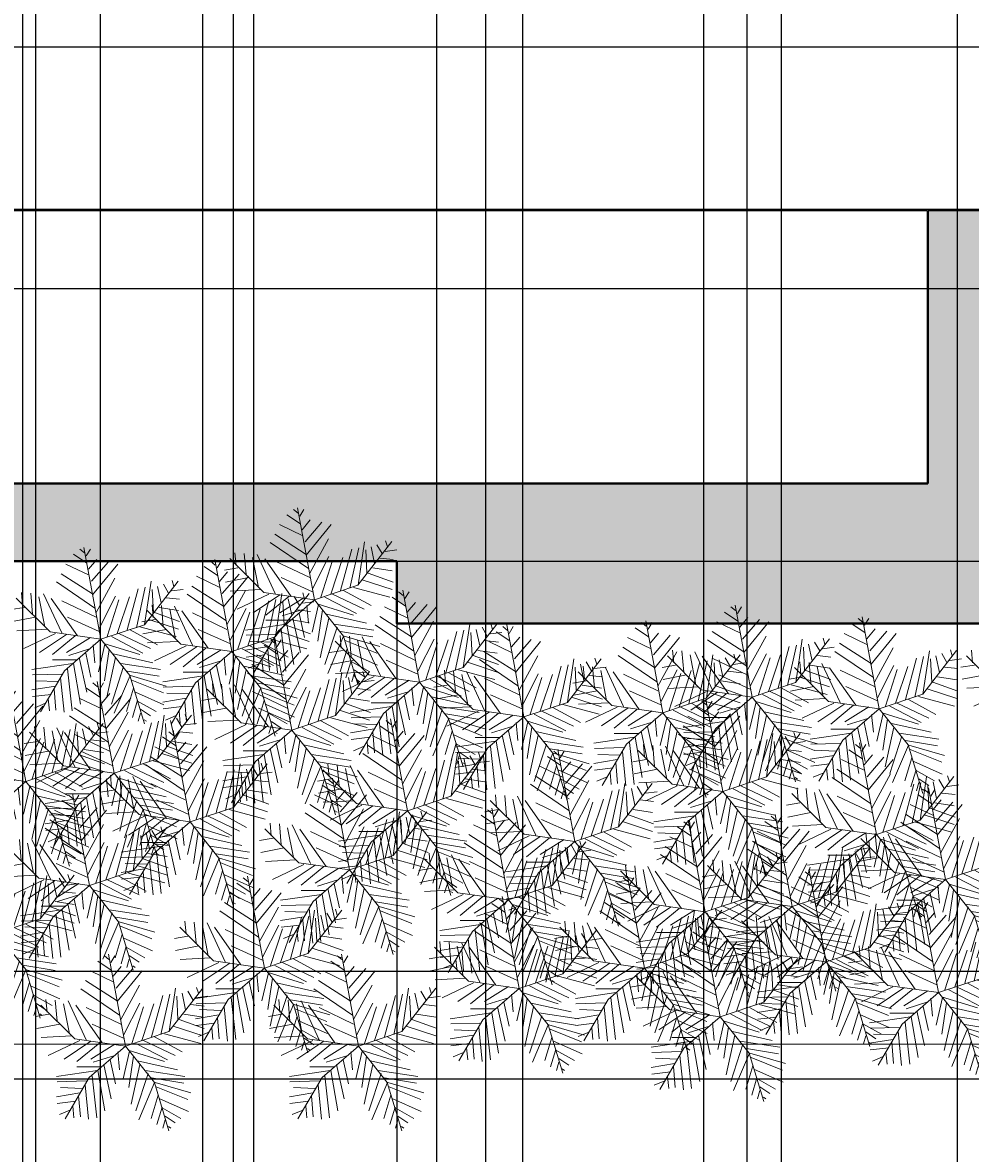
# Model space of a CAD drawing. Units: inches. Extents: x 818 to 1898, y 976 to 2364.
# Tile 38 of 96: x 1512 to 1622, y 1277 to 1409. Entities that reach past the tile are written whole.
import ezdxf

# ---------------------------------------------------------------- set-up
doc = ezdxf.new("R2010")
doc.units = ezdxf.units.IN
doc.header["$LTSCALE"] = 5
doc.header["$MEASUREMENT"] = 0
for name, color, linetype, lineweight in [('A-ANNO-DIMS', 2, 'Continuous', 18), ('A-DOOR', 3, 'Continuous', 25), ('A-WALL', 7, 'Continuous', 40), ('L-PLNT-BEDS', 94, 'Continuous', 18)]:
    doc.layers.add(name, color=color, linetype=linetype, lineweight=lineweight)
doc.layers.add('A-WALL-PATT', color=251, linetype='Continuous', lineweight=13, true_color=0x636466)
doc.layers.add('L-PLNT', color=116, linetype='Continuous', lineweight=13, true_color=0x136734)
doc.styles.get("Standard").update_dxf_attribs({"font": 'arial.ttf'})
doc.dimstyles.get("Standard").update_dxf_attribs({"dimtxt": 0.18, "dimasz": 0.18, "dimexe": 0.18, "dimexo": 0.0625, "dimgap": 0.09, "dimtad": 0, "dimtih": 1, "dimtoh": 1, "dimdec": 4, "dimzin": 0, "dimdsep": 46, "dimtxsty": 'Standard', "dimcen": 0.09, "dimadec": 0, "dimazin": 0, "dimtfac": 1, "dimtdec": 4, "dimtofl": 0, "dimtmove": 0, "dimatfit": 3, "dimfxl": 1, "dimtolj": 1, "dimtzin": 0, "dimarcsym": 0})

# ---------------------------------------------------------------- blocks, each defined once
blk = doc.blocks.new('SHRUB-ACCENT')
for p, q in [((8.8, 18.63), (7.25, 19.67)), ((8.53, 19.84), (7.99, 20.28)), ((10.44, 9.82), (8.47, 20.47)), ((8.74, 19.5), (9.21, 20.28)), ((9.08, 17.24), (6.37, 18.54)), ((9.01, 17.93), (9.96, 19.06)), ((9.35, 16.54), (11.31, 18.8)), ((9.48, 14.98), (12.39, 18.54)), ((9.48, 15.07), (5.82, 17.41)), ((9.75, 13.42), (5.28, 16.46)), ((9.89, 12.9), (12.06, 16.89)), ((14.56, 11.16), (15.58, 15.85)), ((15.49, 11.5), (19.41, 16.55)), ((15.51, 11.51), (16.25, 16.54)), ((17, 15.94), (17.41, 14.03)), ((17.68, 16.2), (18.29, 15.16)), ((18.69, 16.63), (18.9, 15.94)), ((4.55, 10.66), (0.62, 14.58)), ((1.35, 13.77), (1.22, 15.24)), ((2.3, 15.16), (2.51, 12.72)), ((3.25, 14.72), (3.93, 11.25)), ((3.79, 15.07), (5.89, 10.55)), ((7.72, 10.21), (4.67, 14.55)), ((10.23, 11.07), (12.12, 14.81)), ((12.33, 10.47), (13.75, 14.72)), ((13.48, 10.9), (14.76, 15.68)), ((16.39, 15.59), (16.53, 12.9)), ((18.02, 14.63), (19.57, 14.46)), ((18.62, 15.42), (19.98, 15.59)), ((1.56, 13.51), (0, 13.25)), ((5.89, 14.29), (9.89, 12.38)), ((11.17, 10.12), (12.53, 14.37)), ((17.2, 13.51), (19.44, 13.16)), ((2.84, 12.38), (0.14, 11.86)), ((6.57, 12.38), (10.23, 10.73)), ((15.98, 12.12), (19.44, 10.99)), ((16.66, 12.9), (19.57, 11.86)), ((4.2, 10.99), (0.68, 10.81)), ((10.44, 9.82), (4.55, 10.66)), ((10.44, 9.82), (15.49, 11.5)), ((13.82, 10.9), (17, 9.16)), ((14.97, 11.25), (19.17, 10.12)), ((5.15, 10.47), (1.49, 8.73)), ((6.43, 10.38), (3.32, 8.3)), ((7.45, 10.21), (4.81, 8.04)), ((10.44, 9.82), (6.23, 6.17)), ((9.21, 10.03), (6.43, 8.3)), ((10.9, 9.25), (10.16, 6.04)), ((10.44, 9.82), (13.8, 5.61)), ((10.77, 9.34), (14.97, 8.04)), ((11.65, 10.12), (15.31, 8.21)), ((12.53, 10.47), (16.19, 8.73)), ((9.21, 8.73), (6.7, 7.95)), ((8.67, 8.21), (9.28, 5.43)), ((9.55, 9.16), (9.75, 7.08)), ((11.38, 8.64), (10.84, 5)), ((11.85, 8.12), (16.46, 7.08)), ((7.18, 6.99), (2.44, 6.3)), ((7.59, 7.43), (4.81, 7.43)), ((7.25, 6.99), (8.06, 2.31)), ((7.92, 7.69), (8.8, 3.69)), ((12.12, 7.69), (11.11, 3.09)), ((13.07, 6.65), (11.65, 2.31)), ((12.73, 6.99), (17.34, 6.3)), ((5.89, 5.78), (2.51, 5.69)), ((6.23, 6.17), (3.43, 1.4)), ((5.76, 5.34), (6.16, 1.35)), ((6.57, 6.39), (7.11, 1.52)), ((13.82, 5.6), (11.99, 1.26)), ((13.48, 6.13), (17.2, 5.52)), ((13.8, 5.61), (15.49, 0)), ((13.88, 5.6), (18.02, 4.39)), ((5.15, 4.39), (2.44, 3.95)), ((5.42, 4.91), (2.91, 5)), ((5.01, 4.04), (5.21, 1.61)), ((14.22, 4.13), (13.41, 1.44)), ((14.02, 5.08), (17.68, 3.61)), ((4.67, 3.43), (2.51, 3.17)), ((4.33, 2.91), (4.47, 1.52)), ((14.7, 2.74), (14.09, 0.74)), ((14.43, 3.69), (17.74, 2.22)), ((14.7, 2.65), (16.86, 1.44)), ((4, 2.39), (2.78, 1.87)), ((15.04, 1.7), (16.19, 0.92)), ((15.04, 1.26), (14.76, 0.31)), ((15.44, 0.48), (15.71, 0.31))]:
    blk.add_line(p, q)
blk = doc.blocks.new('*D65')
at = {"layer": 'A-ANNO-DIMS', "color": 0, "lineweight": -2, "ltscale": 5, "transparency": 16777216}
for p, q in [((1430.73, 1346.02), (1430.73, 975.66)), ((1714.73, 1346.02), (1714.73, 975.66)), ((1430.91, 975.84), (1572.44, 975.84)), ((1714.55, 975.84), (1573.02, 975.84))]:
    blk.add_line(p, q, dxfattribs=at)
at = {"layer": 'A-ANNO-DIMS', "color": 0, "ltscale": 5, "transparency": 16777216}
for points in [[(1430.91, 975.87), (1430.91, 975.81), (1430.73, 975.84)], [(1714.55, 975.87), (1714.55, 975.81), (1714.73, 975.84)]]:
    blk.add_solid(points, dxfattribs=at)
at = {"layer": 'Defpoints', "color": 0, "ltscale": 5, "transparency": 16777216}
for p in [(1430.73, 1346.08), (1714.73, 1346.08), (1714.73, 975.84)]:
    blk.add_point(p, dxfattribs=at)
at = {"layer": 'A-ANNO-DIMS', "color": 0, "ltscale": 5, "transparency": 16777216, "insert": (1572.73, 975.84), "char_height": 0.18, "attachment_point": 5}
blk.add_mtext('\\A1;284', dxfattribs=at)
blk = doc.blocks.new('*D101')
at = {"layer": 'A-ANNO-DIMS', "color": 0, "lineweight": -2, "ltscale": 5, "transparency": 16777216}
for p, q in [((1507.3, 1071.12), (1507.3, 2363.87)), ((1565.48, 1071.12), (1565.48, 2363.87)), ((1507.48, 2363.69), (1536, 2363.69)), ((1565.3, 2363.69), (1536.78, 2363.69))]:
    blk.add_line(p, q, dxfattribs=at)
at = {"layer": 'A-ANNO-DIMS', "color": 0, "ltscale": 5, "transparency": 16777216}
for points in [[(1507.48, 2363.72), (1507.48, 2363.66), (1507.3, 2363.69)], [(1565.3, 2363.72), (1565.3, 2363.66), (1565.48, 2363.69)]]:
    blk.add_solid(points, dxfattribs=at)
at = {"layer": 'Defpoints', "color": 0, "ltscale": 5, "transparency": 16777216}
for p in [(1565.48, 2363.69), (1507.3, 1071.06), (1565.48, 1071.06)]:
    blk.add_point(p, dxfattribs=at)
at = {"layer": 'A-ANNO-DIMS', "color": 0, "ltscale": 5, "transparency": 16777216, "insert": (1536.39, 2363.69), "char_height": 0.18, "attachment_point": 5}
blk.add_mtext('\\A1;58.19', dxfattribs=at)
blk = doc.blocks.new('*D102')
at = {"layer": 'A-ANNO-DIMS', "color": 0, "lineweight": -2, "ltscale": 5, "transparency": 16777216}
for p, q in [((1565.48, 1071.12), (1565.48, 2363.87)), ((1626.57, 1071.12), (1626.57, 2363.87)), ((1565.66, 2363.69), (1595.63, 2363.69)), ((1626.39, 2363.69), (1596.42, 2363.69))]:
    blk.add_line(p, q, dxfattribs=at)
at = {"layer": 'A-ANNO-DIMS', "color": 0, "ltscale": 5, "transparency": 16777216}
for points in [[(1565.66, 2363.72), (1565.66, 2363.66), (1565.48, 2363.69)], [(1626.39, 2363.72), (1626.39, 2363.66), (1626.57, 2363.69)]]:
    blk.add_solid(points, dxfattribs=at)
at = {"layer": 'Defpoints', "color": 0, "ltscale": 5, "transparency": 16777216}
for p in [(1626.57, 2363.69), (1565.48, 1071.06), (1626.57, 1071.06)]:
    blk.add_point(p, dxfattribs=at)
at = {"layer": 'A-ANNO-DIMS', "color": 0, "ltscale": 5, "transparency": 16777216, "insert": (1596.03, 2363.69), "char_height": 0.18, "attachment_point": 5}
blk.add_mtext('\\A1;61.09', dxfattribs=at)
blk = doc.blocks.new('*D112')
at = {"layer": 'A-ANNO-DIMS', "color": 0, "lineweight": -2, "ltscale": 5, "transparency": 16777216}
for p, q in [((1135.27, 1405.71), (1897.92, 1405.71)), ((1897.74, 1405.53), (1897.74, 1396.48)), ((1897.74, 1387.07), (1897.74, 1396.12)), ((1135.27, 1386.89), (1897.92, 1386.89))]:
    blk.add_line(p, q, dxfattribs=at)
at = {"layer": 'A-ANNO-DIMS', "color": 0, "ltscale": 5, "transparency": 16777216}
for points in [[(1897.71, 1405.53), (1897.77, 1405.53), (1897.74, 1405.71)], [(1897.71, 1387.07), (1897.77, 1387.07), (1897.74, 1386.89)]]:
    blk.add_solid(points, dxfattribs=at)
at = {"layer": 'Defpoints', "color": 0, "ltscale": 5, "transparency": 16777216}
for p in [(1135.21, 1405.71), (1135.21, 1386.89), (1897.74, 1386.89)]:
    blk.add_point(p, dxfattribs=at)
at = {"layer": 'A-ANNO-DIMS', "color": 0, "ltscale": 5, "transparency": 16777216, "insert": (1897.74, 1396.3), "char_height": 0.18, "attachment_point": 5}
blk.add_mtext('\\A1;18.824', dxfattribs=at)
blk = doc.blocks.new('*D113')
at = {"layer": 'A-ANNO-DIMS', "color": 0, "lineweight": -2, "ltscale": 5, "transparency": 16777216}
for p, q in [((1430.79, 1346.08), (1897.92, 1346.08)), ((1897.74, 1345.9), (1897.74, 1316.26)), ((1897.74, 1286.26), (1897.74, 1315.9)), ((1430.79, 1286.08), (1897.92, 1286.08))]:
    blk.add_line(p, q, dxfattribs=at)
at = {"layer": 'A-ANNO-DIMS', "color": 0, "ltscale": 5, "transparency": 16777216}
for points in [[(1897.71, 1345.9), (1897.77, 1345.9), (1897.74, 1346.08)], [(1897.71, 1286.26), (1897.77, 1286.26), (1897.74, 1286.08)]]:
    blk.add_solid(points, dxfattribs=at)
at = {"layer": 'Defpoints', "color": 0, "ltscale": 5, "transparency": 16777216}
for p in [(1430.73, 1346.08), (1897.74, 1346.08), (1430.73, 1286.08)]:
    blk.add_point(p, dxfattribs=at)
at = {"layer": 'A-ANNO-DIMS', "color": 0, "ltscale": 5, "transparency": 16777216, "insert": (1897.74, 1316.08), "char_height": 0.18, "attachment_point": 5}
blk.add_mtext('\\A1;60', dxfattribs=at)
blk = doc.blocks.new('*D115')
at = {"layer": 'A-ANNO-DIMS', "color": 0, "lineweight": -2, "ltscale": 5, "transparency": 16777216}
for p, q in [((1766.29, 1377.66), (818.03, 1377.66)), ((818.21, 1377.48), (818.21, 1338.26)), ((818.21, 1298.68), (818.21, 1337.9)), ((1766.29, 1298.5), (818.03, 1298.5))]:
    blk.add_line(p, q, dxfattribs=at)
at = {"layer": 'A-ANNO-DIMS', "color": 0, "ltscale": 5, "transparency": 16777216}
for points in [[(818.18, 1377.48), (818.24, 1377.48), (818.21, 1377.66)], [(818.18, 1298.68), (818.24, 1298.68), (818.21, 1298.5)]]:
    blk.add_solid(points, dxfattribs=at)
at = {"layer": 'Defpoints', "color": 0, "ltscale": 5, "transparency": 16777216}
for p in [(818.21, 1377.66), (1766.35, 1377.66), (1766.35, 1298.5)]:
    blk.add_point(p, dxfattribs=at)
at = {"layer": 'A-ANNO-DIMS', "color": 0, "ltscale": 5, "transparency": 16777216, "insert": (818.21, 1338.08), "char_height": 0.18, "attachment_point": 5}
blk.add_mtext('\\A1;79.15', dxfattribs=at)
blk = doc.blocks.new('*D116')
at = {"layer": 'A-ANNO-DIMS', "color": 0, "lineweight": -2, "ltscale": 5, "transparency": 16777216}
for p, q in [((1766.29, 1456.81), (818.03, 1456.81)), ((818.21, 1456.63), (818.21, 1417.41)), ((818.21, 1377.84), (818.21, 1417.05)), ((1766.29, 1377.66), (818.03, 1377.66))]:
    blk.add_line(p, q, dxfattribs=at)
at = {"layer": 'A-ANNO-DIMS', "color": 0, "ltscale": 5, "transparency": 16777216}
for points in [[(818.18, 1456.63), (818.24, 1456.63), (818.21, 1456.81)], [(818.18, 1377.84), (818.24, 1377.84), (818.21, 1377.66)]]:
    blk.add_solid(points, dxfattribs=at)
at = {"layer": 'Defpoints', "color": 0, "ltscale": 5, "transparency": 16777216}
for p in [(818.21, 1456.81), (1766.35, 1456.81), (1766.35, 1377.66)]:
    blk.add_point(p, dxfattribs=at)
at = {"layer": 'A-ANNO-DIMS', "color": 0, "ltscale": 5, "transparency": 16777216, "insert": (818.21, 1417.23), "char_height": 0.18, "attachment_point": 5}
blk.add_mtext('\\A1;79.15', dxfattribs=at)
blk = doc.blocks.new('*D171')
at = {"layer": 'A-ANNO-DIMS', "color": 0, "lineweight": -2, "ltscale": 5, "transparency": 16777216}
for p, q in [((1616.66, 1386.69), (818.03, 1386.69)), ((818.21, 1386.51), (818.21, 1371.06)), ((818.21, 1355.26), (818.21, 1370.7)), ((1616.66, 1355.08), (818.03, 1355.08))]:
    blk.add_line(p, q, dxfattribs=at)
at = {"layer": 'A-ANNO-DIMS', "color": 0, "ltscale": 5, "transparency": 16777216}
for points in [[(818.18, 1386.51), (818.24, 1386.51), (818.21, 1386.69)], [(818.18, 1355.26), (818.24, 1355.26), (818.21, 1355.08)]]:
    blk.add_solid(points, dxfattribs=at)
at = {"layer": 'Defpoints', "color": 0, "ltscale": 5, "transparency": 16777216}
for p in [(818.21, 1386.69), (1616.73, 1386.69), (1616.73, 1355.08)]:
    blk.add_point(p, dxfattribs=at)
at = {"layer": 'A-ANNO-DIMS', "color": 0, "ltscale": 5, "transparency": 16777216, "insert": (818.21, 1370.88), "char_height": 0.18, "attachment_point": 5}
blk.add_mtext('\\A1;31.61', dxfattribs=at)
blk = doc.blocks.new('*D172')
at = {"layer": 'A-ANNO-DIMS', "color": 0, "lineweight": -2, "ltscale": 5, "transparency": 16777216}
for p, q in [((1616.66, 1416.69), (818.03, 1416.69)), ((818.21, 1416.51), (818.21, 1401.87)), ((818.21, 1386.87), (818.21, 1401.5)), ((1616.66, 1386.69), (818.03, 1386.69))]:
    blk.add_line(p, q, dxfattribs=at)
at = {"layer": 'A-ANNO-DIMS', "color": 0, "ltscale": 5, "transparency": 16777216}
for points in [[(818.18, 1416.51), (818.24, 1416.51), (818.21, 1416.69)], [(818.18, 1386.87), (818.24, 1386.87), (818.21, 1386.69)]]:
    blk.add_solid(points, dxfattribs=at)
at = {"layer": 'Defpoints', "color": 0, "ltscale": 5, "transparency": 16777216}
for p in [(818.21, 1416.69), (1616.73, 1416.69), (1616.73, 1386.69)]:
    blk.add_point(p, dxfattribs=at)
at = {"layer": 'A-ANNO-DIMS', "color": 0, "ltscale": 5, "transparency": 16777216, "insert": (818.21, 1401.69), "char_height": 0.18, "attachment_point": 5}
blk.add_mtext('\\A1;30', dxfattribs=at)
blk = doc.blocks.new('*D177')
at = {"layer": 'A-ANNO-DIMS', "color": 0, "lineweight": -2, "ltscale": 5, "transparency": 16777216}
for p, q in [((1559.73, 1647.52), (1559.73, 975.66)), ((1569.73, 1647.52), (1569.73, 975.66)), ((1559.91, 975.84), (1564.52, 975.84)), ((1569.55, 975.84), (1564.94, 975.84))]:
    blk.add_line(p, q, dxfattribs=at)
at = {"layer": 'A-ANNO-DIMS', "color": 0, "ltscale": 5, "transparency": 16777216}
for points in [[(1559.91, 975.87), (1559.91, 975.81), (1559.73, 975.84)], [(1569.55, 975.87), (1569.55, 975.81), (1569.73, 975.84)]]:
    blk.add_solid(points, dxfattribs=at)
at = {"layer": 'Defpoints', "color": 0, "ltscale": 5, "transparency": 16777216}
for p in [(1559.73, 1647.58), (1569.73, 1647.58), (1569.73, 975.84)]:
    blk.add_point(p, dxfattribs=at)
at = {"layer": 'A-ANNO-DIMS', "color": 0, "ltscale": 5, "transparency": 16777216, "insert": (1564.73, 975.84), "char_height": 0.18, "attachment_point": 5}
blk.add_mtext('\\A1;10', dxfattribs=at)
blk = doc.blocks.new('*D180')
at = {"layer": 'A-ANNO-DIMS', "color": 0, "lineweight": -2, "ltscale": 5, "transparency": 16777216}
for p, q in [((1599.73, 1639.52), (1599.73, 975.66)), ((1669.73, 1639.52), (1669.73, 975.66)), ((1599.91, 975.84), (1634.51, 975.84)), ((1669.55, 975.84), (1634.94, 975.84))]:
    blk.add_line(p, q, dxfattribs=at)
at = {"layer": 'A-ANNO-DIMS', "color": 0, "ltscale": 5, "transparency": 16777216}
for points in [[(1599.91, 975.87), (1599.91, 975.81), (1599.73, 975.84)], [(1669.55, 975.87), (1669.55, 975.81), (1669.73, 975.84)]]:
    blk.add_solid(points, dxfattribs=at)
at = {"layer": 'Defpoints', "color": 0, "ltscale": 5, "transparency": 16777216}
for p in [(1599.73, 1639.58), (1669.73, 1639.58), (1669.73, 975.84)]:
    blk.add_point(p, dxfattribs=at)
at = {"layer": 'A-ANNO-DIMS', "color": 0, "ltscale": 5, "transparency": 16777216, "insert": (1634.73, 975.84), "char_height": 0.18, "attachment_point": 5}
blk.add_mtext('\\A1;70', dxfattribs=at)
blk = doc.blocks.new('*D182')
at = {"layer": 'A-ANNO-DIMS', "color": 0, "lineweight": -2, "ltscale": 5, "transparency": 16777216}
for p, q in [((1463.73, 1687.02), (1463.73, 975.66)), ((1559.73, 1687.02), (1559.73, 975.66)), ((1463.91, 975.84), (1511.51, 975.84)), ((1559.55, 975.84), (1511.94, 975.84))]:
    blk.add_line(p, q, dxfattribs=at)
at = {"layer": 'A-ANNO-DIMS', "color": 0, "ltscale": 5, "transparency": 16777216}
for points in [[(1463.91, 975.87), (1463.91, 975.81), (1463.73, 975.84)], [(1559.55, 975.87), (1559.55, 975.81), (1559.73, 975.84)]]:
    blk.add_solid(points, dxfattribs=at)
at = {"layer": 'Defpoints', "color": 0, "ltscale": 5, "transparency": 16777216}
for p in [(1463.73, 1687.08), (1559.73, 1687.08), (1559.73, 975.84)]:
    blk.add_point(p, dxfattribs=at)
at = {"layer": 'A-ANNO-DIMS', "color": 0, "ltscale": 5, "transparency": 16777216, "insert": (1511.73, 975.84), "char_height": 0.18, "attachment_point": 5}
blk.add_mtext('\\A1;96', dxfattribs=at)
blk = doc.blocks.new('*D192')
at = {"layer": 'A-ANNO-DIMS', "color": 0, "lineweight": -2, "ltscale": 5, "transparency": 16777216}
for p, q in [((1555.13, 1338.8), (1555.13, 975.66)), ((1660.31, 1338.8), (1660.31, 975.66)), ((1555.31, 975.84), (1607.27, 975.84)), ((1660.13, 975.84), (1608.18, 975.84))]:
    blk.add_line(p, q, dxfattribs=at)
at = {"layer": 'A-ANNO-DIMS', "color": 0, "ltscale": 5, "transparency": 16777216}
for points in [[(1555.31, 975.87), (1555.31, 975.81), (1555.13, 975.84)], [(1660.13, 975.87), (1660.13, 975.81), (1660.31, 975.84)]]:
    blk.add_solid(points, dxfattribs=at)
at = {"layer": 'Defpoints', "color": 0, "ltscale": 5, "transparency": 16777216}
for p in [(1555.13, 1338.87), (1660.31, 1338.87), (1660.31, 975.84)]:
    blk.add_point(p, dxfattribs=at)
at = {"layer": 'A-ANNO-DIMS', "color": 0, "ltscale": 5, "transparency": 16777216, "insert": (1607.72, 975.84), "char_height": 0.18, "attachment_point": 5}
blk.add_mtext('\\A1;105.18', dxfattribs=at)
blk = doc.blocks.new('*D198')
at = {"layer": 'A-ANNO-DIMS', "color": 0, "lineweight": -2, "ltscale": 5, "transparency": 16777216}
for p, q in [((1741.84, 1545.02), (1741.84, 975.66)), ((1430.73, 1346.02), (1430.73, 975.66)), ((1430.91, 975.84), (1585.91, 975.84)), ((1741.66, 975.84), (1586.66, 975.84))]:
    blk.add_line(p, q, dxfattribs=at)
at = {"layer": 'A-ANNO-DIMS', "color": 0, "ltscale": 5, "transparency": 16777216}
for points in [[(1430.91, 975.87), (1430.91, 975.81), (1430.73, 975.84)], [(1741.66, 975.87), (1741.66, 975.81), (1741.84, 975.84)]]:
    blk.add_solid(points, dxfattribs=at)
at = {"layer": 'Defpoints', "color": 0, "ltscale": 5, "transparency": 16777216}
for p in [(1741.84, 1545.08), (1430.73, 1346.08), (1741.84, 975.84)]:
    blk.add_point(p, dxfattribs=at)
at = {"layer": 'A-ANNO-DIMS', "color": 0, "ltscale": 5, "transparency": 16777216, "insert": (1586.28, 975.84), "char_height": 0.18, "attachment_point": 5}
blk.add_mtext('\\A1;311.1', dxfattribs=at)
blk = doc.blocks.new('*D199')
at = {"layer": 'A-ANNO-DIMS', "color": 0, "lineweight": -2, "ltscale": 5, "transparency": 16777216}
for p, q in [((1559.79, 1687.08), (1897.92, 1687.08)), ((1897.74, 1686.9), (1897.74, 1513.15)), ((1897.74, 1339.05), (1897.74, 1512.79)), ((1660.38, 1338.87), (1897.92, 1338.87))]:
    blk.add_line(p, q, dxfattribs=at)
at = {"layer": 'A-ANNO-DIMS', "color": 0, "ltscale": 5, "transparency": 16777216}
for points in [[(1897.71, 1686.9), (1897.77, 1686.9), (1897.74, 1687.08)], [(1897.71, 1339.05), (1897.77, 1339.05), (1897.74, 1338.87)]]:
    blk.add_solid(points, dxfattribs=at)
at = {"layer": 'Defpoints', "color": 0, "ltscale": 5, "transparency": 16777216}
for p in [(1559.73, 1687.08), (1897.74, 1687.08), (1660.31, 1338.87)]:
    blk.add_point(p, dxfattribs=at)
at = {"layer": 'A-ANNO-DIMS', "color": 0, "ltscale": 5, "transparency": 16777216, "insert": (1897.74, 1512.97), "char_height": 0.18, "attachment_point": 5}
blk.add_mtext('\\A1;348.2', dxfattribs=at)
blk = doc.blocks.new('*D214')
at = {"layer": 'A-ANNO-DIMS', "color": 0, "lineweight": -2, "ltscale": 5, "transparency": 16777216}
for p, q in [((1511.73, 1687.02), (1511.73, 975.66)), ((1714.73, 1687.02), (1714.73, 975.66)), ((1511.91, 975.84), (1612.93, 975.84)), ((1714.55, 975.84), (1613.52, 975.84))]:
    blk.add_line(p, q, dxfattribs=at)
at = {"layer": 'A-ANNO-DIMS', "color": 0, "ltscale": 5, "transparency": 16777216}
for points in [[(1511.91, 975.87), (1511.91, 975.81), (1511.73, 975.84)], [(1714.55, 975.87), (1714.55, 975.81), (1714.73, 975.84)]]:
    blk.add_solid(points, dxfattribs=at)
at = {"layer": 'Defpoints', "color": 0, "ltscale": 5, "transparency": 16777216}
for p in [(1511.73, 1687.08), (1714.73, 1687.08), (1714.73, 975.84)]:
    blk.add_point(p, dxfattribs=at)
at = {"layer": 'A-ANNO-DIMS', "color": 0, "ltscale": 5, "transparency": 16777216, "insert": (1613.23, 975.84), "char_height": 0.18, "attachment_point": 5}
blk.add_mtext('\\A1;203', dxfattribs=at)
blk = doc.blocks.new('*D219')
at = {"layer": 'A-ANNO-DIMS', "color": 0, "lineweight": -2, "ltscale": 5, "transparency": 16777216}
for p, q in [((1595.73, 1696.02), (1595.73, 975.66)), ((1599.73, 1696.02), (1599.73, 975.66)), ((1595.91, 975.84), (1597.57, 975.84)), ((1599.55, 975.84), (1597.88, 975.84))]:
    blk.add_line(p, q, dxfattribs=at)
at = {"layer": 'A-ANNO-DIMS', "color": 0, "ltscale": 5, "transparency": 16777216}
for points in [[(1595.91, 975.87), (1595.91, 975.81), (1595.73, 975.84)], [(1599.55, 975.87), (1599.55, 975.81), (1599.73, 975.84)]]:
    blk.add_solid(points, dxfattribs=at)
at = {"layer": 'Defpoints', "color": 0, "ltscale": 5, "transparency": 16777216}
for p in [(1595.73, 1696.08), (1599.73, 1696.08), (1599.73, 975.84)]:
    blk.add_point(p, dxfattribs=at)
at = {"layer": 'A-ANNO-DIMS', "color": 0, "ltscale": 5, "transparency": 16777216, "insert": (1597.73, 975.84), "char_height": 0.18, "attachment_point": 5}
blk.add_mtext('\\A1;4', dxfattribs=at)
blk = doc.blocks.new('*D224')
at = {"layer": 'A-ANNO-DIMS', "color": 0, "lineweight": -2, "ltscale": 5, "transparency": 16777216}
for p, q in [((1520.73, 1837.52), (1520.73, 975.66)), ((1532.59, 1837.52), (1532.59, 975.66)), ((1520.91, 975.84), (1526.2, 975.84)), ((1532.41, 975.84), (1527.11, 975.84))]:
    blk.add_line(p, q, dxfattribs=at)
at = {"layer": 'A-ANNO-DIMS', "color": 0, "ltscale": 5, "transparency": 16777216}
for points in [[(1520.91, 975.87), (1520.91, 975.81), (1520.73, 975.84)], [(1532.41, 975.87), (1532.41, 975.81), (1532.59, 975.84)]]:
    blk.add_solid(points, dxfattribs=at)
at = {"layer": 'Defpoints', "color": 0, "ltscale": 5, "transparency": 16777216}
for p in [(1520.73, 1837.58), (1532.59, 1837.58), (1532.59, 975.84)]:
    blk.add_point(p, dxfattribs=at)
at = {"layer": 'A-ANNO-DIMS', "color": 0, "ltscale": 5, "transparency": 16777216, "insert": (1526.66, 975.84), "char_height": 0.18, "attachment_point": 5}
blk.add_mtext('\\A1;11.868', dxfattribs=at)
blk = doc.blocks.new('*D226')
at = {"layer": 'A-ANNO-DIMS', "color": 0, "lineweight": -2, "ltscale": 5, "transparency": 16777216}
for p, q in [((1536.17, 1774.47), (1536.17, 975.66)), ((1520.73, 1773.02), (1520.73, 975.66)), ((1520.91, 975.84), (1527.99, 975.84)), ((1535.99, 975.84), (1528.9, 975.84))]:
    blk.add_line(p, q, dxfattribs=at)
at = {"layer": 'A-ANNO-DIMS', "color": 0, "ltscale": 5, "transparency": 16777216}
for points in [[(1520.91, 975.87), (1520.91, 975.81), (1520.73, 975.84)], [(1535.99, 975.87), (1535.99, 975.81), (1536.17, 975.84)]]:
    blk.add_solid(points, dxfattribs=at)
at = {"layer": 'Defpoints', "color": 0, "ltscale": 5, "transparency": 16777216}
for p in [(1536.17, 1774.53), (1520.73, 1773.08), (1536.17, 975.84)]:
    blk.add_point(p, dxfattribs=at)
at = {"layer": 'A-ANNO-DIMS', "color": 0, "ltscale": 5, "transparency": 16777216, "insert": (1528.45, 975.84), "char_height": 0.18, "attachment_point": 5}
blk.add_mtext('\\A1;15.445', dxfattribs=at)
blk = doc.blocks.new('*D229')
at = {"layer": 'A-ANNO-DIMS', "color": 0, "lineweight": -2, "ltscale": 5, "transparency": 16777216}
for p, q in [((1599.73, 2044.02), (1599.73, 975.66)), ((1620.14, 2036.06), (1620.14, 975.66)), ((1599.91, 975.84), (1609.47, 975.84)), ((1619.96, 975.84), (1610.4, 975.84))]:
    blk.add_line(p, q, dxfattribs=at)
at = {"layer": 'A-ANNO-DIMS', "color": 0, "ltscale": 5, "transparency": 16777216}
for points in [[(1599.91, 975.87), (1599.91, 975.81), (1599.73, 975.84)], [(1619.96, 975.87), (1619.96, 975.81), (1620.14, 975.84)]]:
    blk.add_solid(points, dxfattribs=at)
at = {"layer": 'Defpoints', "color": 0, "ltscale": 5, "transparency": 16777216}
for p in [(1599.73, 2044.08), (1620.14, 2036.12), (1620.14, 975.84)]:
    blk.add_point(p, dxfattribs=at)
at = {"layer": 'A-ANNO-DIMS', "color": 0, "ltscale": 5, "transparency": 16777216, "insert": (1609.93, 975.84), "char_height": 0.18, "attachment_point": 5}
blk.add_mtext('\\A1;20.416', dxfattribs=at)
blk = doc.blocks.new('*D242')
at = {"layer": 'A-ANNO-DIMS', "color": 0, "lineweight": -2, "ltscale": 5, "transparency": 16777216}
for p, q in [((1488.26, 1948.6), (1488.26, 975.66)), ((1513.23, 1948.6), (1513.23, 975.66)), ((1488.44, 975.84), (1500.35, 975.84)), ((1513.05, 975.84), (1501.14, 975.84))]:
    blk.add_line(p, q, dxfattribs=at)
at = {"layer": 'A-ANNO-DIMS', "color": 0, "ltscale": 5, "transparency": 16777216}
for points in [[(1488.44, 975.87), (1488.44, 975.81), (1488.26, 975.84)], [(1513.05, 975.87), (1513.05, 975.81), (1513.23, 975.84)]]:
    blk.add_solid(points, dxfattribs=at)
at = {"layer": 'Defpoints', "color": 0, "ltscale": 5, "transparency": 16777216}
for p in [(1488.26, 1948.66), (1513.23, 1948.66), (1513.23, 975.84)]:
    blk.add_point(p, dxfattribs=at)
at = {"layer": 'A-ANNO-DIMS', "color": 0, "ltscale": 5, "transparency": 16777216, "insert": (1500.74, 975.84), "char_height": 0.18, "attachment_point": 5}
blk.add_mtext('\\A1;24.97', dxfattribs=at)
blk = doc.blocks.new('*D243')
at = {"layer": 'A-ANNO-DIMS', "color": 0, "lineweight": -2, "ltscale": 5, "transparency": 16777216}
for p, q in [((1451.77, 2020.02), (1451.77, 975.66)), ((1590.73, 2020.02), (1590.73, 975.66)), ((1451.95, 975.84), (1520.79, 975.84)), ((1590.55, 975.84), (1521.7, 975.84))]:
    blk.add_line(p, q, dxfattribs=at)
at = {"layer": 'A-ANNO-DIMS', "color": 0, "ltscale": 5, "transparency": 16777216}
for points in [[(1451.95, 975.87), (1451.95, 975.81), (1451.77, 975.84)], [(1590.55, 975.87), (1590.55, 975.81), (1590.73, 975.84)]]:
    blk.add_solid(points, dxfattribs=at)
at = {"layer": 'Defpoints', "color": 0, "ltscale": 5, "transparency": 16777216}
for p in [(1451.77, 2020.08), (1590.73, 2020.08), (1590.73, 975.84)]:
    blk.add_point(p, dxfattribs=at)
at = {"layer": 'A-ANNO-DIMS', "color": 0, "ltscale": 5, "transparency": 16777216, "insert": (1521.25, 975.84), "char_height": 0.18, "attachment_point": 5}
blk.add_mtext('\\A1;138.96', dxfattribs=at)
blk = doc.blocks.new('*D253')
at = {"layer": 'A-ANNO-DIMS', "color": 0, "lineweight": -2, "ltscale": 5, "transparency": 16777216}
for p, q in [((1485.12, 2053.02), (1485.12, 975.66)), ((1538.52, 2053.02), (1538.52, 975.66)), ((1485.3, 975.84), (1511.42, 975.84)), ((1538.34, 975.84), (1512.21, 975.84))]:
    blk.add_line(p, q, dxfattribs=at)
at = {"layer": 'A-ANNO-DIMS', "color": 0, "ltscale": 5, "transparency": 16777216}
for points in [[(1485.3, 975.87), (1485.3, 975.81), (1485.12, 975.84)], [(1538.34, 975.87), (1538.34, 975.81), (1538.52, 975.84)]]:
    blk.add_solid(points, dxfattribs=at)
at = {"layer": 'Defpoints', "color": 0, "ltscale": 5, "transparency": 16777216}
for p in [(1485.12, 2053.08), (1538.52, 2053.08), (1538.52, 975.84)]:
    blk.add_point(p, dxfattribs=at)
at = {"layer": 'A-ANNO-DIMS', "color": 0, "ltscale": 5, "transparency": 16777216, "insert": (1511.82, 975.84), "char_height": 0.18, "attachment_point": 5}
blk.add_mtext('\\A1;53.39', dxfattribs=at)

msp = doc.modelspace()

# ---------------------------------------------------------------- hatches: boundary and pattern name
at = {"layer": 'A-WALL-PATT', "ltscale": 5}
h = msp.add_hatch(color=256, dxfattribs=at)
h.dxf.hatch_style = 1
h.paths.add_polyline_path([(1714.7251, 1521.0782), (1705.7252, 1521.0782), (1705.7252, 1467.0782), (1654.7252, 1467.0782), (1654.7252, 1463.0782), (1705.7252, 1463.0782), (1705.7252, 1355.0782), (1622.7252, 1355.0782), (1622.7252, 1379.0782), (1622.7252, 1386.6857), (1616.7251, 1386.6857), (1616.7251, 1355.0782), (1490.9163, 1355.0782), (1490.9163, 1346.0782), (1544.7605, 1346.0782), (1544.6132, 1346.8783), (1544.6729, 1346.84), (1544.6299, 1346.7874), (1544.7605, 1346.0782), (1555.1299, 1346.0782), (1555.1299, 1341.5528), (1556.1599, 1340.8639), (1556.5281, 1338.8654), (1660.3141, 1338.8654), (1660.3141, 1346.0782), (1705.7252, 1346.0782), (1705.7252, 1345.0768), (1705.8704, 1344.58), (1705.7252, 1344.3933), (1705.7252, 1334.9904), (1705.8704, 1334.4936), (1705.7252, 1334.3068), (1705.7252, 1316.2253), (1707.3573, 1316.7694), (1707.3847, 1316.8046), (1707.3807, 1316.7771), (1705.7252, 1316.2253), (1705.7252, 1314.1392), (1705.7252, 1312.0957), (1705.8703, 1312.0739), (1705.7252, 1311.8873), (1705.7252, 1310.7121), (1706.5603, 1307.9282), (1707.8887, 1307.1831), (1714.7251, 1307.1831), (1714.7251, 1346.0782)])

# ---------------------------------------------------------------- linework, layer by layer
at = {"layer": 'A-DOOR'}
msp.add_line((1622.7252, 1386.6857), (1616.7251, 1386.6857), dxfattribs=at)
at = {"layer": 'A-WALL'}
for p, q in [((1616.7251, 1386.6857), (1616.7251, 1355.0782)), ((1439.7252, 1355.0782), (1616.7251, 1355.0782)), ((1430.7251, 1346.0782), (1555.1299, 1346.0782))]:
    msp.add_line(p, q, dxfattribs=at)
at = {"layer": 'A-WALL', "ltscale": 5}
msp.add_lwpolyline([(1660.3141, 1346.0782), (1660.3141, 1338.8654), (1555.1299, 1338.8654), (1555.1299, 1346.0782)], dxfattribs=at)
at = {"layer": 'L-PLNT'}
for p, q in [((1543.678, 1351.6453), (1543.1362, 1352.0794)), ((1545.5824, 1341.6169), (1543.6193, 1352.2735)), ((1543.8812, 1351.298), (1544.3554, 1352.0794)), ((1544.2198, 1349.0404), (1541.5108, 1350.3428)), ((1543.9489, 1350.4297), (1542.3912, 1351.4716)), ((1544.1521, 1349.7352), (1545.1004, 1350.8638)), ((1544.4907, 1348.3459), (1546.4549, 1350.6034)), ((1544.6263, 1346.7829), (1547.5385, 1350.3428)), ((1544.6263, 1346.8699), (1540.969, 1349.2141)), ((1544.8972, 1345.2202), (1540.4272, 1348.259)), ((1545.0325, 1344.6991), (1547.1999, 1348.6933)), ((1550.6302, 1343.2995), (1554.5563, 1348.3474)), ((1550.654, 1343.31), (1551.399, 1348.3459)), ((1552.1438, 1347.7381), (1552.5503, 1345.8279)), ((1552.8212, 1347.9985), (1553.4306, 1346.9566)), ((1553.8371, 1348.4326), (1554.0401, 1347.7381)), ((1539.6932, 1342.4582), (1535.7671, 1346.3843)), ((1536.499, 1345.5675), (1536.3637, 1347.0435)), ((1537.4473, 1346.9566), (1537.6503, 1344.5256)), ((1538.3953, 1346.5225), (1539.0727, 1343.0496)), ((1538.9371, 1346.8699), (1541.0367, 1342.3548)), ((1545.3713, 1342.8759), (1547.2676, 1346.6094)), ((1547.4708, 1342.2681), (1548.893, 1346.5225)), ((1548.6221, 1342.7022), (1549.9089, 1347.4777)), ((1549.7057, 1342.9626), (1550.7216, 1347.6513)), ((1551.5343, 1347.3907), (1551.6699, 1344.6991)), ((1553.1597, 1346.4357), (1554.7175, 1346.2621)), ((1553.7694, 1347.217), (1555.1239, 1347.3907)), ((1536.7022, 1345.3069), (1535.1445, 1345.0465)), ((1542.8653, 1342.0077), (1539.8177, 1346.3488)), ((1541.0367, 1346.0884), (1545.0325, 1344.1782)), ((1546.3193, 1341.9207), (1547.6739, 1346.1751)), ((1552.347, 1345.3069), (1554.5819, 1344.9597)), ((1537.9891, 1344.1782), (1535.2801, 1343.6572)), ((1541.714, 1344.1782), (1545.3713, 1342.5285)), ((1551.1279, 1343.9178), (1554.5819, 1342.789)), ((1551.8052, 1344.6991), (1554.7175, 1343.6572)), ((1539.3436, 1342.789), (1535.8219, 1342.6153)), ((1545.5824, 1341.6169), (1539.6932, 1342.4582)), ((1545.5824, 1341.6169), (1550.6302, 1343.2995)), ((1548.9607, 1342.7022), (1552.1438, 1340.9657)), ((1550.1122, 1343.0496), (1554.311, 1341.9207)), ((1555.8776, 1342.0871), (1555.3358, 1342.5212)), ((1557.7819, 1332.0587), (1555.8189, 1342.7153)), ((1556.0808, 1341.7397), (1556.5549, 1342.5212)), ((1540.2916, 1342.2681), (1536.6346, 1340.5316)), ((1541.5785, 1342.1812), (1538.4632, 1340.0973)), ((1542.5944, 1342.0077), (1539.9531, 1339.8369)), ((1545.5824, 1341.6169), (1541.3758, 1337.9712)), ((1544.3554, 1341.834), (1541.5785, 1340.0973)), ((1545.5824, 1341.6169), (1548.9476, 1337.4104)), ((1545.9131, 1341.1392), (1550.1122, 1339.8369)), ((1546.7935, 1341.9207), (1550.4507, 1340.0106)), ((1547.6739, 1342.2681), (1551.3311, 1340.5316)), ((1556.1485, 1340.8715), (1554.5908, 1341.9134)), ((1556.3517, 1340.177), (1557.3, 1341.3056)), ((1544.3554, 1340.5316), (1541.8494, 1339.7501)), ((1543.8136, 1340.0106), (1544.423, 1337.2322)), ((1544.6939, 1340.9657), (1544.8972, 1338.8819)), ((1546.0484, 1341.0525), (1545.3036, 1337.84)), ((1546.5226, 1340.4447), (1545.9808, 1336.7981)), ((1546.9967, 1339.9238), (1551.602, 1338.8819)), ((1556.4194, 1339.4822), (1553.7104, 1340.7846)), ((1556.6903, 1338.7877), (1558.6545, 1341.0452)), ((1556.8258, 1337.2247), (1559.7381, 1340.7846)), ((1542.3235, 1338.795), (1537.5826, 1338.1004)), ((1542.7299, 1339.2291), (1539.9531, 1339.2291)), ((1542.3912, 1338.795), (1543.2041, 1334.1065)), ((1543.0685, 1339.4897), (1543.9489, 1335.4957)), ((1547.2676, 1339.4897), (1546.2517, 1334.8879)), ((1547.8771, 1338.795), (1552.4824, 1338.1004)), ((1557.0967, 1335.6619), (1552.6268, 1338.7007)), ((1556.8258, 1337.3117), (1553.1686, 1339.6559)), ((1557.2321, 1335.1409), (1559.3995, 1339.1351)), ((1562.8298, 1333.7413), (1566.7559, 1338.7892)), ((1562.8535, 1333.7518), (1563.5986, 1338.7877)), ((1566.0367, 1338.8744), (1566.2397, 1338.1799)), ((1541.0367, 1337.5794), (1537.6503, 1337.4926)), ((1541.3758, 1337.9712), (1538.5714, 1333.2038)), ((1541.714, 1338.1872), (1542.2558, 1333.325)), ((1548.2157, 1338.4478), (1546.7935, 1334.1065)), ((1548.9607, 1337.4059), (1547.132, 1333.0645)), ((1548.6986, 1336.0093), (1548.5632, 1337.4853)), ((1548.6221, 1337.9268), (1552.347, 1337.319)), ((1548.9476, 1337.4104), (1550.6302, 1331.8016)), ((1549.0285, 1337.4059), (1553.1597, 1336.1903)), ((1549.6469, 1337.3984), (1549.8499, 1334.9674)), ((1551.1367, 1337.3117), (1553.2362, 1332.7966)), ((1560.8217, 1333.144), (1562.1085, 1337.9195)), ((1561.9053, 1333.4044), (1562.9212, 1338.0931)), ((1563.7339, 1337.8325), (1563.8695, 1335.1409)), ((1564.3434, 1338.1799), (1564.7498, 1336.2697)), ((1565.0207, 1338.4403), (1565.6302, 1337.3984)), ((1565.969, 1337.6588), (1567.3235, 1337.8325)), ((1540.2916, 1336.1903), (1537.5826, 1335.7562)), ((1540.5627, 1336.7112), (1538.0568, 1336.7981)), ((1540.9013, 1337.1453), (1541.3076, 1333.1513)), ((1551.8928, 1332.9), (1547.9667, 1336.8261)), ((1549.3671, 1335.9299), (1548.5544, 1333.2382)), ((1549.1639, 1336.8848), (1552.8212, 1335.4088)), ((1550.5949, 1336.9643), (1551.2723, 1333.4914)), ((1555.0649, 1332.4494), (1552.0173, 1336.7906)), ((1553.2362, 1336.5302), (1557.2321, 1334.62)), ((1557.5709, 1333.3177), (1559.4672, 1337.0512)), ((1558.5189, 1332.3625), (1559.8734, 1336.6169)), ((1559.6704, 1332.7099), (1561.0926, 1336.9643)), ((1565.3593, 1336.8775), (1566.9171, 1336.7039)), ((1539.8177, 1335.2351), (1537.6503, 1334.9747)), ((1539.4789, 1334.7143), (1539.6145, 1333.325)), ((1540.1563, 1335.8429), (1540.3595, 1333.4119)), ((1548.9018, 1335.7487), (1547.3441, 1335.4883)), ((1550.1887, 1334.62), (1547.4796, 1334.099)), ((1549.5703, 1335.4957), (1552.8888, 1334.0197)), ((1553.9136, 1334.62), (1557.5709, 1332.9703)), ((1564.0048, 1335.1409), (1566.9171, 1334.099)), ((1564.5466, 1335.7487), (1566.7815, 1335.4015)), ((1539.1404, 1334.1932), (1537.9212, 1333.6723)), ((1549.8412, 1334.5406), (1549.2316, 1332.5435)), ((1549.8412, 1334.4538), (1552.0085, 1333.2382)), ((1550.1798, 1333.4987), (1551.3311, 1332.7172)), ((1557.7819, 1332.0587), (1562.8298, 1333.7413)), ((1562.3117, 1333.4914), (1566.5106, 1332.3625)), ((1563.3275, 1334.3596), (1566.7815, 1333.2307)), ((1551.5432, 1333.2307), (1548.0214, 1333.0571)), ((1552.4912, 1332.7099), (1548.8341, 1330.9734)), ((1550.1798, 1333.0645), (1549.9089, 1332.1094)), ((1550.5861, 1332.2831), (1550.857, 1332.1094)), ((1553.7781, 1332.6229), (1550.6628, 1330.5391)), ((1557.7819, 1332.0587), (1551.8928, 1332.9)), ((1554.794, 1332.4494), (1552.1526, 1330.2787)), ((1557.7819, 1332.0587), (1553.5754, 1328.413)), ((1556.5549, 1332.2758), (1553.7781, 1330.5391)), ((1557.7819, 1332.0587), (1561.1472, 1327.8522)), ((1558.993, 1332.3625), (1562.6503, 1330.4524)), ((1559.8734, 1332.7099), (1563.5307, 1330.9734)), ((1561.1603, 1333.144), (1564.3434, 1331.4075)), ((1556.5549, 1330.9734), (1554.049, 1330.1919)), ((1556.8935, 1331.4075), (1557.0967, 1329.3237)), ((1558.248, 1331.4943), (1557.5032, 1328.2818)), ((1558.1127, 1331.581), (1562.3117, 1330.2787)), ((1558.7221, 1330.8865), (1558.1803, 1327.2399)), ((1554.9295, 1329.6709), (1552.1526, 1329.6709)), ((1555.2681, 1329.9315), (1556.1485, 1325.9375)), ((1556.0131, 1330.4524), (1556.6226, 1327.674)), ((1559.4672, 1329.9315), (1558.4512, 1325.3297)), ((1559.1963, 1330.3656), (1563.8016, 1329.3237)), ((1554.5231, 1329.2368), (1549.7822, 1328.5422)), ((1553.5754, 1328.413), (1550.771, 1323.6456)), ((1553.9136, 1328.629), (1554.4554, 1323.7668)), ((1554.5908, 1329.2368), (1555.4036, 1324.5483)), ((1560.4152, 1328.8896), (1558.993, 1324.5483)), ((1560.0767, 1329.2368), (1564.682, 1328.5422)), ((1560.8217, 1328.3685), (1564.5466, 1327.7607)), ((1553.2362, 1328.0212), (1549.8499, 1327.9344)), ((1552.7623, 1327.1529), (1550.2563, 1327.2399)), ((1553.1009, 1327.5871), (1553.5072, 1323.5931)), ((1561.1603, 1327.8477), (1559.3316, 1323.5063)), ((1561.1472, 1327.8522), (1562.8298, 1322.2434)), ((1561.2281, 1327.8477), (1565.3593, 1326.6321)), ((1561.3635, 1327.3266), (1565.0207, 1325.8506)), ((1552.4912, 1326.6321), (1549.7822, 1326.198)), ((1552.0173, 1325.6769), (1549.8499, 1325.4165)), ((1552.3559, 1326.2847), (1552.5591, 1323.8537)), ((1561.5667, 1326.3716), (1560.754, 1323.68)), ((1561.7699, 1325.9375), (1565.0884, 1324.4615)), ((1551.3399, 1324.635), (1550.1208, 1324.1141)), ((1551.6785, 1325.1561), (1551.8141, 1323.7668)), ((1562.0408, 1324.9824), (1561.4312, 1322.9853)), ((1562.0408, 1324.8956), (1564.208, 1323.68)), ((1562.3794, 1323.5063), (1562.1085, 1322.5512)), ((1562.3794, 1323.9405), (1563.5307, 1323.159)), ((1562.7857, 1322.7249), (1563.0566, 1322.5512))]:
    msp.add_line(p, q, dxfattribs=at)
at = {"layer": 'L-PLNT-BEDS', "ltscale": 5}
for points in [[(1430.7251, 1286.0782), (1701.3688, 1286.0782, 0.41421356), (1713.3688, 1298.0782), (1713.3688, 1307.1831)], [(1430.7251, 1290.0782), (1701.3688, 1290.0782, 0.41421356), (1709.3688, 1298.0782), (1709.3688, 1307.1831)]]:
    msp.add_lwpolyline(points, format="xyb", dxfattribs=at)

# ---------------------------------------------------------------- block references
at = {"layer": 'L-PLNT'}
for p in [(1510.3731, 1327.216), (1525.5407, 1325.7952), (1585.9085, 1320.5145), (1620.5869, 1320.5352), (1559.4308, 1318.2176), (1575.5464, 1318.6912), (1600.6677, 1319.1648), (1532.5164, 1316.6784), (1511.9006, 1311.6818), (1501.674, 1310.7268), (1582.5221, 1309.5744), (1545.9222, 1307.3249), (1520.705, 1306.0381), (1565.3556, 1303.7729), (1600.3441, 1304.5585), (1539.2171, 1300.4656), (1509.055, 1298.6736), (1608.3357, 1299.349), (1557.6723, 1296.9836), (1590.5777, 1296.2267), (1580.4571, 1295.6032), (1498.2864, 1293.1169), (1594.5059, 1289.8017), (1529.3326, 1289.0913), (1573.4134, 1289.0913), (1558.8915, 1286.7382), (1607.5406, 1286.2497), (1582.2178, 1283.4476), (1513.217, 1280.0457), (1540.2343, 1280.0457)]:
    msp.add_blockref('SHRUB-ACCENT', p, dxfattribs=at)

# ---------------------------------------------------------------- dimensions: what is measured, and where the dimension line sits
at = {"layer": 'A-ANNO-DIMS', "ltscale": 5}
for base, p1, p2, override, picture, middle in [((1565.4835, 2363.6929), (1507.2982, 1071.0552), (1565.4835, 1071.0552), {"dimdec": 2, "dimlfac": 1, "dimrnd": 0, "dimzin": 0, "dimdsep": 46, "dimlunit": 2}, '*D101', (1536.3908, 2363.6929)), ((1626.5748, 2363.6929), (1565.4835, 1071.0552), (1626.5748, 1071.0552), {"dimdec": 2, "dimlfac": 1, "dimrnd": 0, "dimzin": 0, "dimdsep": 46, "dimlunit": 2}, '*D102', (1596.0291, 2363.6929)), ((1538.5155, 975.8433), (1485.1216, 2053.0782), (1538.5155, 2053.0782), {"dimdec": 2, "dimlfac": 1, "dimrnd": 0, "dimzin": 0, "dimdsep": 46, "dimlunit": 2}, '*D253', (1511.8185, 975.8433)), ((1620.14159, 975.84326), (1599.72515, 2044.07824), (1620.14159, 2036.1182), {"dimdec": 3, "dimlfac": 1, "dimrnd": 0, "dimzin": 0, "dimdsep": 46, "dimlunit": 2}, '*D229', (1609.93337, 975.84326)), ((1590.7251, 975.8433), (1451.7698, 2020.0782), (1590.7251, 2020.0782), {"dimdec": 2, "dimlfac": 1, "dimrnd": 0, "dimzin": 0, "dimdsep": 46, "dimlunit": 2}, '*D243', (1521.2475, 975.8433)), ((1513.2306, 975.8433), (1488.2586, 1948.6602), (1513.2306, 1948.6602), {"dimdec": 2, "dimlfac": 1, "dimrnd": 0, "dimzin": 0, "dimdsep": 46, "dimlunit": 2}, '*D242', (1500.7446, 975.8433)), ((1532.593, 975.8433), (1520.7251, 1837.5823), (1532.593, 1837.5823), {"dimdec": 3, "dimlfac": 1, "dimrnd": 0, "dimzin": 0, "dimdsep": 46, "dimlunit": 2}, '*D224', (1526.6591, 975.8433)), ((1536.1698, 975.8433), (1520.7251, 1773.0782), (1536.1698, 1774.5283), {"dimdec": 3, "dimlfac": 1, "dimrnd": 0, "dimzin": 0, "dimdsep": 46, "dimlunit": 2}, '*D226', (1528.4475, 975.8433)), ((1599.7251, 975.8433), (1595.7251, 1696.0782), (1599.7251, 1696.0782), {"dimdec": 0, "dimlfac": 1, "dimrnd": 0, "dimzin": 0, "dimdsep": 46, "dimlunit": 2}, '*D219', (1597.7251, 975.8433)), ((1559.7251, 975.8433), (1463.7251, 1687.0782), (1559.7251, 1687.0782), {"dimdec": 0, "dimlfac": 1, "dimrnd": 0, "dimzin": 0, "dimdsep": 46, "dimlunit": 2}, '*D182', (1511.7251, 975.8433)), ((1714.7251, 975.8433), (1511.7251, 1687.0782), (1714.7251, 1687.0782), {"dimdec": 0, "dimlfac": 1, "dimrnd": 0, "dimzin": 0, "dimdsep": 46, "dimlunit": 2}, '*D214', (1613.2251, 975.8433)), ((1569.7251, 975.8433), (1559.7251, 1647.5782), (1569.7251, 1647.5782), {"dimdec": 0, "dimlfac": 1, "dimrnd": 0, "dimzin": 0, "dimdsep": 46, "dimlunit": 2}, '*D177', (1564.7251, 975.8433)), ((1669.7251, 975.8433), (1599.7251, 1639.5782), (1669.7251, 1639.5782), {"dimdec": 0, "dimlfac": 1, "dimrnd": 0, "dimzin": 0, "dimdsep": 46, "dimlunit": 2}, '*D180', (1634.7251, 975.8433)), ((1741.8409, 975.8433), (1430.7251, 1346.0782), (1741.8409, 1545.0782), {"dimdec": 1, "dimlfac": 1, "dimrnd": 0, "dimzin": 0, "dimdsep": 46, "dimlunit": 2}, '*D198', (1586.283, 975.8433)), ((1714.7251, 975.8433), (1430.7251, 1346.0782), (1714.7251, 1346.0782), {"dimdec": 0, "dimlfac": 1, "dimrnd": 0, "dimzin": 0, "dimdsep": 46, "dimlunit": 2}, '*D65', (1572.7251, 975.8433)), ((1660.3141, 975.8433), (1555.1299, 1338.8654), (1660.3141, 1338.8654), {"dimdec": 2, "dimlfac": 1, "dimrnd": 0, "dimzin": 0, "dimdsep": 46, "dimlunit": 2}, '*D192', (1607.722, 975.8433))]:
    dim = msp.add_linear_dim(base=base, p1=p1, p2=p2, dimstyle='Standard', override=override, dxfattribs=at)
    dim.commit()
    dim.dimension.update_dxf_attribs({"geometry": picture, "text_midpoint": middle})
for base, p1, p2, override, picture, middle in [((1897.736, 1687.0782), (1660.3141, 1338.8654), (1559.7251, 1687.0782), {"dimdec": 1, "dimlfac": 1, "dimrnd": 0, "dimzin": 0, "dimdsep": 46, "dimlunit": 2}, '*D199', (1897.736, 1512.9718)), ((818.2059, 1456.8088), (1766.3524, 1377.6564), (1766.3524, 1456.8088), {"dimdec": 2, "dimlfac": 1, "dimrnd": 0, "dimzin": 0, "dimdsep": 46, "dimlunit": 2}, '*D116', (818.2059, 1417.2326)), ((818.2059, 1416.6857), (1616.7251, 1386.6857), (1616.7251, 1416.6857), {"dimdec": 0, "dimlfac": 1, "dimrnd": 0, "dimzin": 0, "dimdsep": 46, "dimlunit": 2}, '*D172', (818.2059, 1401.6857)), ((1897.736, 1386.8851), (1135.2058, 1405.7088), (1135.2058, 1386.8851), {"dimdec": 3, "dimlfac": 1, "dimrnd": 0, "dimzin": 0, "dimdsep": 46, "dimlunit": 2}, '*D112', (1897.736, 1396.297)), ((818.2059, 1386.6857), (1616.7251, 1355.0782), (1616.7251, 1386.6857), {"dimdec": 2, "dimlfac": 1, "dimrnd": 0, "dimzin": 0, "dimdsep": 46, "dimlunit": 2}, '*D171', (818.2059, 1370.882)), ((818.2059, 1377.6564), (1766.3524, 1298.5041), (1766.3524, 1377.6564), {"dimdec": 2, "dimlfac": 1, "dimrnd": 0, "dimzin": 0, "dimdsep": 46, "dimlunit": 2}, '*D115', (818.2059, 1338.0803)), ((1897.736, 1346.0782), (1430.7251, 1286.0782), (1430.7251, 1346.0782), {"dimdec": 0, "dimlfac": 1, "dimrnd": 0, "dimzin": 0, "dimdsep": 46, "dimlunit": 2}, '*D113', (1897.736, 1316.0782))]:
    dim = msp.add_linear_dim(base=base, p1=p1, p2=p2, angle=90, dimstyle='Standard', override=override, dxfattribs=at)
    dim.commit()
    dim.dimension.update_dxf_attribs({"geometry": picture, "text_midpoint": middle})

doc.saveas('drawing.dxf')
